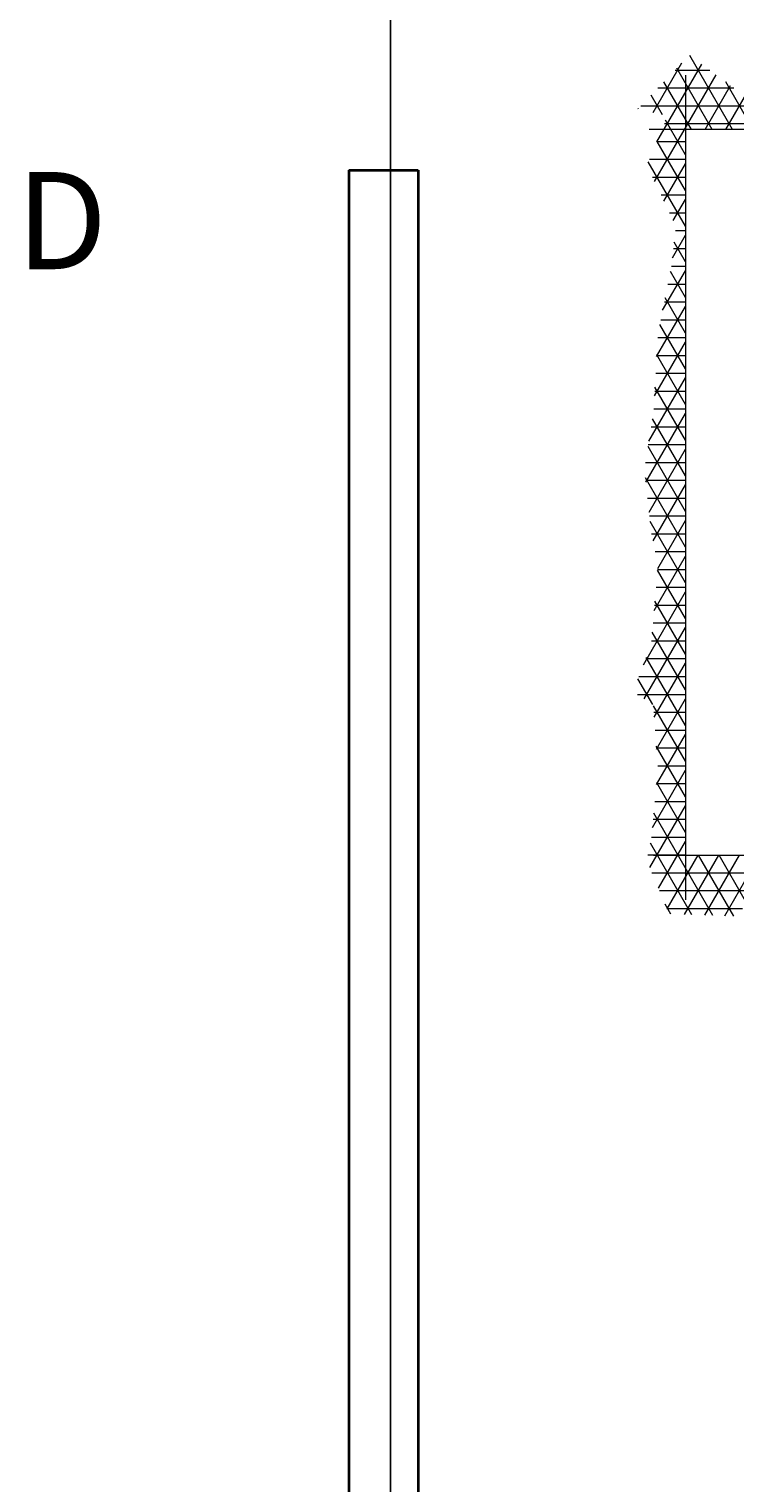
# Model space of a CAD drawing. Units: inches. Extents: x 3731 to 4318, y 1310 to 2388.
# Tile 16 of 57: x 4086 to 4137, y 1397 to 1502. Entities that reach past the tile are written whole.
import ezdxf

# ---------------------------------------------------------------- set-up
doc = ezdxf.new("R2010")
doc.units = ezdxf.units.IN
for name, color, linetype, lineweight in [('A-ANNO-DIMS', 2, 'Continuous', 18), ('A-ANNO-TEXT', 7, 'Continuous', 18), ('A-FURN', 8, 'Continuous', 13), ('A-WALL', 7, 'Continuous', 35)]:
    doc.layers.add(name, color=color, linetype=linetype, lineweight=lineweight)
doc.styles.get("Standard").update_dxf_attribs({"font": 'arial.ttf'})
doc.dimstyles.get("Standard").update_dxf_attribs({"dimtxt": 0.18, "dimasz": 0.18, "dimexe": 0.18, "dimexo": 0.0625, "dimgap": 0.09, "dimtad": 0, "dimtih": 1, "dimtoh": 1, "dimdec": 4, "dimzin": 0, "dimdsep": 46, "dimtxsty": 'Standard', "dimcen": 0.09, "dimadec": 0, "dimazin": 0, "dimtfac": 1, "dimtdec": 4, "dimtofl": 0, "dimtmove": 0, "dimatfit": 3, "dimfxl": 1, "dimtolj": 1, "dimtzin": 0, "dimarcsym": 0})

# ---------------------------------------------------------------- blocks, each defined once
blk = doc.blocks.new('A$C200C7901')
for p, q in [((2.3121, 1.6596), (2.3121, 0.0201)), ((1.0407, 0.0275), (1.0407, 0.4323)), ((2.4073, 0.0839), (0.9625, 0.0839))]:
    blk.add_line(p, q)
at = {"linetype": 'ByBlock'}
for p, q in [((2.3224, 0.0468), (2.3224, 1.6627)), ((2.3224, 0.0468), (2.3224, 1.6627)), ((2.3537, 0.0056), (2.3537, 1.634)), ((2.3537, 0.0056), (2.3537, 1.634)), ((0.9344, 0.153), (1.0407, 0.2144)), ((0.9344, 0.153), (1.0407, 0.2144)), ((1.0099, 0.0251), (1.0099, 0.2117)), ((1.0099, 0.0251), (1.0099, 0.2117)), ((0.9355, 0.1176), (1.0407, 0.1783)), ((0.9355, 0.1176), (1.0407, 0.1783)), ((0.9474, 0.0512), (0.9474, 0.1835)), ((0.9474, 0.0512), (0.9474, 0.1835)), ((0.9602, 0.1893), (1.0407, 0.1428)), ((0.9602, 0.1893), (1.0407, 0.1428)), ((0.9787, 0.0381), (0.9787, 0.1976)), ((0.9787, 0.0381), (0.9787, 0.1976)), ((2.3121, 0.2026), (2.3953, 0.1545)), ((2.3121, 0.2026), (2.3953, 0.1545)), ((2.3121, 0.1546), (2.3755, 0.1912)), ((2.3121, 0.1546), (2.3755, 0.1912)), ((0.9339, 0.1684), (1.0407, 0.1067)), ((0.9339, 0.1684), (1.0407, 0.1067)), ((2.3121, 0.1665), (2.4419, 0.0916)), ((2.3121, 0.1665), (2.4419, 0.0916)), ((2.3121, 0.1185), (2.3891, 0.163)), ((2.3121, 0.1185), (2.3891, 0.163)), ((2.3849, 0.0355), (2.3849, 0.1686)), ((2.3849, 0.0355), (2.3849, 0.1686)), ((0.935, 0.1316), (1.114, 0.0283)), ((0.935, 0.1316), (1.114, 0.0283)), ((0.9366, 0.0822), (1.0407, 0.1422)), ((0.9366, 0.0822), (1.0407, 0.1422)), ((2.2208, 0.0297), (2.4078, 0.1377)), ((2.2208, 0.0297), (2.4078, 0.1377)), ((2.3121, 0.1304), (2.4193, 0.0685)), ((2.3121, 0.1304), (2.4193, 0.0685)), ((0.9463, 0.0516), (1.0407, 0.1061)), ((0.9463, 0.0516), (1.0407, 0.1061)), ((2.2903, 0.0337), (2.4265, 0.1124)), ((2.2903, 0.0337), (2.4265, 0.1124)), ((2.4162, 0.0655), (2.4162, 0.1264)), ((2.4162, 0.0655), (2.4162, 0.1264)), ((0.9362, 0.0948), (1.0616, 0.0225)), ((0.9362, 0.0948), (1.0616, 0.0225)), ((0.9826, 0.0365), (1.0647, 0.0839)), ((0.9826, 0.0365), (1.0647, 0.0839)), ((1.0189, 0.0214), (1.1272, 0.0839)), ((1.0189, 0.0214), (1.1272, 0.0839)), ((1.0412, 0.0179), (1.0412, 0.0839)), ((1.0412, 0.0179), (1.0412, 0.0839)), ((1.0724, 0.0243), (1.0724, 0.0839)), ((1.0724, 0.0243), (1.0724, 0.0839)), ((1.0801, 0.0839), (1.1675, 0.0335)), ((1.0801, 0.0839), (1.1675, 0.0335)), ((1.0891, 0.0259), (1.1897, 0.0839)), ((1.0891, 0.0259), (1.1897, 0.0839)), ((1.1037, 0.0273), (1.1037, 0.0839)), ((1.1037, 0.0273), (1.1037, 0.0839)), ((1.1349, 0.0303), (1.1349, 0.0839)), ((1.1349, 0.0303), (1.1349, 0.0839)), ((1.1426, 0.0839), (1.2313, 0.0327)), ((1.1426, 0.0839), (1.2313, 0.0327)), ((1.1642, 0.0331), (1.2522, 0.0839)), ((1.1642, 0.0331), (1.2522, 0.0839)), ((1.1662, 0.0333), (1.1662, 0.0839)), ((1.1662, 0.0333), (1.1662, 0.0839)), ((1.1974, 0.0351), (1.1974, 0.0839)), ((1.1974, 0.0351), (1.1974, 0.0839)), ((1.2051, 0.0839), (1.3023, 0.0278)), ((1.2051, 0.0839), (1.3023, 0.0278)), ((1.2266, 0.033), (1.3147, 0.0839)), ((1.2266, 0.033), (1.3147, 0.0839)), ((1.2287, 0.0329), (1.2287, 0.0839)), ((1.2287, 0.0329), (1.2287, 0.0839)), ((1.2599, 0.0308), (1.2599, 0.0839)), ((1.2599, 0.0308), (1.2599, 0.0839)), ((1.2676, 0.0839), (1.3871, 0.015)), ((1.2676, 0.0839), (1.3871, 0.015)), ((1.2824, 0.0292), (1.3772, 0.0839)), ((1.2824, 0.0292), (1.3772, 0.0839)), ((1.2912, 0.0286), (1.2912, 0.0839)), ((1.2912, 0.0286), (1.2912, 0.0839)), ((1.3146, 0.0117), (1.4397, 0.0839)), ((1.3146, 0.0117), (1.4397, 0.0839)), ((1.3224, 0), (1.3224, 0.0839)), ((1.3224, 0), (1.3224, 0.0839)), ((1.3301, 0.0839), (1.4312, 0.0256)), ((1.3301, 0.0839), (1.4312, 0.0256)), ((1.3537, 0.0022), (1.3537, 0.0839)), ((1.3537, 0.0022), (1.3537, 0.0839)), ((1.3743, 0.0101), (1.5022, 0.0839)), ((1.3743, 0.0101), (1.5022, 0.0839)), ((1.3849, 0.0141), (1.3849, 0.0839)), ((1.3849, 0.0141), (1.3849, 0.0839)), ((1.3926, 0.0839), (1.4856, 0.0302)), ((1.3926, 0.0839), (1.4856, 0.0302)), ((1.4162, 0.0243), (1.4162, 0.0839)), ((1.4162, 0.0243), (1.4162, 0.0839)), ((1.4474, 0.027), (1.4474, 0.0839)), ((1.4474, 0.027), (1.4474, 0.0839)), ((1.4551, 0.0839), (1.54, 0.0349)), ((1.4551, 0.0839), (1.54, 0.0349)), ((1.4693, 0.0288), (1.5647, 0.0839)), ((1.4693, 0.0288), (1.5647, 0.0839)), ((1.4787, 0.0296), (1.4787, 0.0839)), ((1.4787, 0.0296), (1.4787, 0.0839)), ((1.5099, 0.0323), (1.5099, 0.0839)), ((1.5099, 0.0323), (1.5099, 0.0839)), ((1.5176, 0.0839), (1.6251, 0.0219)), ((1.5176, 0.0839), (1.6251, 0.0219)), ((1.5412, 0.035), (1.5412, 0.0839)), ((1.5412, 0.035), (1.5412, 0.0839)), ((1.5427, 0.0351), (1.6272, 0.0839)), ((1.5427, 0.0351), (1.6272, 0.0839)), ((1.5724, 0.0308), (1.5724, 0.0839)), ((1.5724, 0.0308), (1.5724, 0.0839)), ((1.5801, 0.0839), (1.7018, 0.0137)), ((1.5801, 0.0839), (1.7018, 0.0137)), ((1.5911, 0.027), (1.6897, 0.0839)), ((1.5911, 0.027), (1.6897, 0.0839)), ((1.6037, 0.0245), (1.6037, 0.0839)), ((1.6037, 0.0245), (1.6037, 0.0839)), ((1.6349, 0.0208), (1.6349, 0.0839)), ((1.6349, 0.0208), (1.6349, 0.0839)), ((1.6416, 0.0201), (1.7522, 0.0839)), ((1.6416, 0.0201), (1.7522, 0.0839)), ((1.6426, 0.0839), (1.7565, 0.0182)), ((1.6426, 0.0839), (1.7565, 0.0182)), ((1.6662, 0.0175), (1.6662, 0.0839)), ((1.6662, 0.0175), (1.6662, 0.0839)), ((1.6944, 0.0145), (1.8147, 0.0839)), ((1.6944, 0.0145), (1.8147, 0.0839)), ((1.6974, 0.0141), (1.6974, 0.0839)), ((1.6974, 0.0141), (1.6974, 0.0839)), ((1.7051, 0.0839), (1.8054, 0.026)), ((1.7051, 0.0839), (1.8054, 0.026)), ((1.7287, 0.0137), (1.7287, 0.0839)), ((1.7287, 0.0137), (1.7287, 0.0839)), ((1.7599, 0.0187), (1.7599, 0.0839)), ((1.7599, 0.0187), (1.7599, 0.0839)), ((1.7659, 0.0197), (1.8772, 0.0839)), ((1.7659, 0.0197), (1.8772, 0.0839)), ((1.7676, 0.0839), (1.8606, 0.0303)), ((1.7676, 0.0839), (1.8606, 0.0303)), ((1.7912, 0.0237), (1.7912, 0.0839)), ((1.7912, 0.0237), (1.7912, 0.0839)), ((1.8224, 0.0281), (1.8224, 0.0839)), ((1.8224, 0.0281), (1.8224, 0.0839)), ((1.8301, 0.0839), (1.9175, 0.0335)), ((1.8301, 0.0839), (1.9175, 0.0335)), ((1.8452, 0.0294), (1.9397, 0.0839)), ((1.8452, 0.0294), (1.9397, 0.0839)), ((1.8537, 0.0299), (1.8537, 0.0839)), ((1.8537, 0.0299), (1.8537, 0.0839)), ((1.8849, 0.0316), (1.8849, 0.0839)), ((1.8849, 0.0316), (1.8849, 0.0839)), ((1.8926, 0.0839), (1.9706, 0.0389)), ((1.8926, 0.0839), (1.9706, 0.0389)), ((1.9146, 0.0333), (2.0022, 0.0839)), ((1.9146, 0.0333), (2.0022, 0.0839)), ((1.9162, 0.0334), (1.9162, 0.0839)), ((1.9162, 0.0334), (1.9162, 0.0839)), ((1.9474, 0.0352), (1.9474, 0.0839)), ((1.9474, 0.0352), (1.9474, 0.0839)), ((1.9551, 0.0839), (2.017, 0.0482)), ((1.9551, 0.0839), (2.017, 0.0482)), ((1.9787, 0.0405), (1.9787, 0.0839)), ((1.9787, 0.0405), (1.9787, 0.0839)), ((1.9953, 0.0438), (2.0647, 0.0839)), ((1.9953, 0.0438), (2.0647, 0.0839)), ((2.0099, 0.0468), (2.0099, 0.0839)), ((2.0099, 0.0468), (2.0099, 0.0839)), ((2.0176, 0.0839), (2.0634, 0.0575)), ((2.0176, 0.0839), (2.0634, 0.0575)), ((2.0412, 0.053), (2.0412, 0.0839)), ((2.0412, 0.053), (2.0412, 0.0839)), ((2.0724, 0.0592), (2.0724, 0.0839)), ((2.0724, 0.0592), (2.0724, 0.0839)), ((2.0801, 0.0839), (2.1147, 0.0639)), ((2.0801, 0.0839), (2.1147, 0.0639)), ((2.0873, 0.0609), (2.1272, 0.0839)), ((2.0873, 0.0609), (2.1272, 0.0839)), ((2.1037, 0.0627), (2.1037, 0.0839)), ((2.1037, 0.0627), (2.1037, 0.0839)), ((2.1349, 0.0662), (2.1349, 0.0839)), ((2.1349, 0.0662), (2.1349, 0.0839)), ((2.1426, 0.0839), (2.2557, 0.0186)), ((2.1426, 0.0839), (2.2557, 0.0186)), ((2.1526, 0.0625), (2.1897, 0.0839)), ((2.1526, 0.0625), (2.1897, 0.0839)), ((2.1662, 0.056), (2.1662, 0.0839)), ((2.1662, 0.056), (2.1662, 0.0839)), ((2.1867, 0.0461), (2.2522, 0.0839)), ((2.1867, 0.0461), (2.2522, 0.0839)), ((2.1974, 0.041), (2.1974, 0.0839)), ((2.1974, 0.041), (2.1974, 0.0839)), ((2.2051, 0.0839), (2.2913, 0.0342)), ((2.2051, 0.0839), (2.2913, 0.0342)), ((2.2287, 0.0259), (2.2287, 0.0839)), ((2.2287, 0.0259), (2.2287, 0.0839)), ((2.2599, 0.0205), (2.2599, 0.0839)), ((2.2599, 0.0205), (2.2599, 0.0839)), ((2.2676, 0.0839), (2.3285, 0.0488)), ((2.2676, 0.0839), (2.3285, 0.0488)), ((2.2912, 0.0341), (2.2912, 0.0839)), ((2.2912, 0.0341), (2.2912, 0.0839)), ((2.3121, 0.0943), (2.3958, 0.046)), ((2.3121, 0.0943), (2.3958, 0.046)), ((2.3417, 0.0273), (2.429, 0.0777)), ((2.3417, 0.0273), (2.429, 0.0777)), ((0.9374, 0.0581), (0.9545, 0.0482)), ((0.9374, 0.0581), (0.9545, 0.0482)), ((1.3048, 0.0264), (1.3494, 0.0006)), ((1.3048, 0.0264), (1.3494, 0.0006)), ((2.338, 0.0433), (2.3723, 0.0235)), ((2.338, 0.0433), (2.3723, 0.0235)), ((2.3476, 0.0017), (2.3488, 0.001)), ((2.3476, 0.0017), (2.3488, 0.001))]:
    blk.add_line(p, q, dxfattribs=at)
blk = doc.blocks.new('*D32')
at = {"layer": 'A-ANNO-DIMS', "color": 0, "lineweight": -2, "transparency": 16777216}
for p, q in [((4269.21, 1592.32), (4269.21, 1310.25)), ((3835.21, 1359.32), (3835.21, 1310.25)), ((3835.39, 1310.43), (4051.92, 1310.43)), ((4269.03, 1310.43), (4052.5, 1310.43))]:
    blk.add_line(p, q, dxfattribs=at)
at = {"layer": 'A-ANNO-DIMS', "color": 0, "transparency": 16777216}
for points in [[(3835.39, 1310.46), (3835.39, 1310.4), (3835.21, 1310.43)], [(4269.03, 1310.46), (4269.03, 1310.4), (4269.21, 1310.43)]]:
    blk.add_solid(points, dxfattribs=at)
at = {"layer": 'Defpoints', "color": 0, "transparency": 16777216}
for p in [(4269.21, 1592.38), (3835.21, 1359.38), (4269.21, 1310.43)]:
    blk.add_point(p, dxfattribs=at)
at = {"layer": 'A-ANNO-DIMS', "color": 0, "transparency": 16777216, "insert": (4052.21, 1310.43), "char_height": 0.18, "attachment_point": 5}
blk.add_mtext('\\A1;434', dxfattribs=at)
blk = doc.blocks.new('*D46')
at = {"layer": 'A-ANNO-DIMS', "color": 0, "lineweight": -2, "transparency": 16777216}
for p, q in [((4112.21, 1854.32), (4112.21, 1310.25)), ((4192.21, 1854.32), (4192.21, 1310.25)), ((4112.39, 1310.43), (4151.99, 1310.43)), ((4192.03, 1310.43), (4152.43, 1310.43))]:
    blk.add_line(p, q, dxfattribs=at)
at = {"layer": 'A-ANNO-DIMS', "color": 0, "transparency": 16777216}
for points in [[(4112.39, 1310.46), (4112.39, 1310.4), (4112.21, 1310.43)], [(4192.03, 1310.46), (4192.03, 1310.4), (4192.21, 1310.43)]]:
    blk.add_solid(points, dxfattribs=at)
at = {"layer": 'Defpoints', "color": 0, "transparency": 16777216}
for p in [(4112.21, 1854.38), (4192.21, 1854.38), (4192.21, 1310.43)]:
    blk.add_point(p, dxfattribs=at)
at = {"layer": 'A-ANNO-DIMS', "color": 0, "transparency": 16777216, "insert": (4152.21, 1310.43), "char_height": 0.18, "attachment_point": 5}
blk.add_mtext('\\A1;80', dxfattribs=at)

msp = doc.modelspace()

# ---------------------------------------------------------------- linework, layer by layer
at = {"layer": 'A-WALL'}
for p, q in [((4109.21, 1491.38), (4114.21, 1491.38)), ((4109.21, 1491.38), (4109.21, 1364.38)), ((4114.21, 1491.38), (4114.21, 1364.38))]:
    msp.add_line(p, q, dxfattribs=at)

# ---------------------------------------------------------------- block references
at = {"layer": 'A-FURN', "xscale": -41.1071563136412, "yscale": 41.1071563136412, "zscale": 41.1071563136412, "rotation": 270}
msp.add_blockref('A$C200C7901', (4130.02, 1399.26), dxfattribs=at)

# ---------------------------------------------------------------- texts
at = {"layer": 'A-ANNO-TEXT', "insert": (4085.24, 1491.24), "char_height": 7, "attachment_point": 1}
msp.add_mtext_dynamic_manual_height_columns('D', width=10.4564, gutter_width=12.5, heights=[0], dxfattribs=at)

# ---------------------------------------------------------------- dimensions: what is measured, and where the dimension line sits
at = {"layer": 'A-ANNO-DIMS'}
for base, p1, p2, picture, middle in [((4192.21, 1310.43), (4112.21, 1854.38), (4192.21, 1854.38), '*D46', (4152.21, 1310.43)), ((4269.21, 1310.43), (3835.21, 1359.38), (4269.21, 1592.38), '*D32', (4052.21, 1310.43))]:
    dim = msp.add_linear_dim(base=base, p1=p1, p2=p2, dimstyle='Standard', override={"dimdec": 0, "dimlfac": 1, "dimrnd": 0, "dimzin": 0, "dimdsep": 46, "dimlunit": 2}, dxfattribs=at)
    dim.commit()
    dim.dimension.update_dxf_attribs({"geometry": picture, "text_midpoint": middle})

doc.saveas('drawing.dxf')
